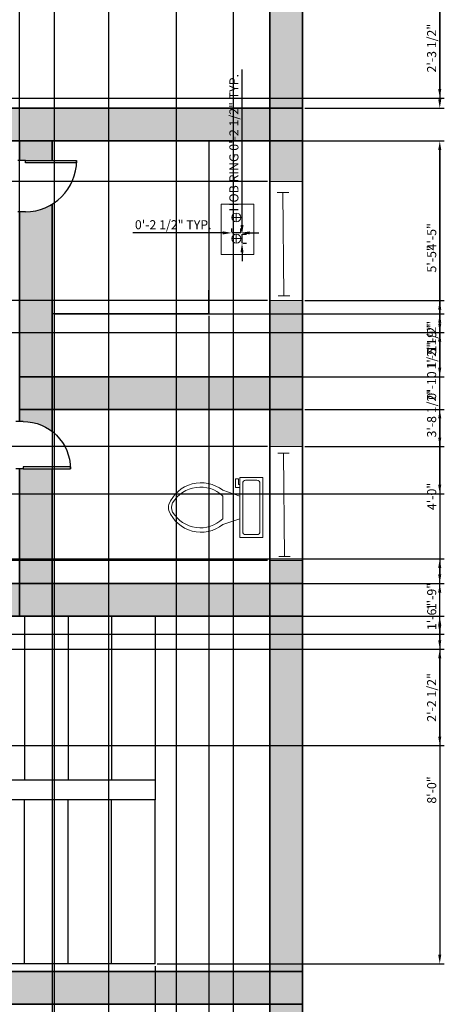
# Model space of a CAD drawing. Units: millimetres. Extents: x 2856 to 3283, y 634 to 1474.
# Tile 7 of 8: x 3165 to 3283, y 1050 to 1321. Entities that reach past the tile are written whole.
import ezdxf

# ---------------------------------------------------------------- set-up
doc = ezdxf.new("R2010")
doc.units = ezdxf.units.MM
for name, color, linetype, lineweight in [('A-ANNO-DIMS', 90, 'Continuous', 18), ('A-EQPM', 140, 'Continuous', 18), ('A-FLOR-CASE', 140, 'Continuous', 25), ('A-FLOR-FIXT', 140, 'Continuous', 18), ('A-WALL-PATT', 2, 'Continuous', 13), ('doors', 10, 'Continuous', 25), ('staircase', 160, 'Continuous', 25), ('walls', 50, 'Continuous', 35), ('windows', 30, 'Continuous', 18)]:
    doc.layers.add(name, color=color, linetype=linetype, lineweight=lineweight)
doc.styles.get("Standard").update_dxf_attribs({"font": 'arial.ttf'})
doc.dimstyles.new('ISO-25', dxfattribs={"dimtxt": 2.5, "dimasz": 2.5, "dimexe": 1.25, "dimexo": 0.625, "dimtad": 1, "dimdec": 0, "dimlunit": 3, "dimtxsty": 'Standard', "dimcen": 2.5, "dimadec": 0, "dimazin": 0, "dimtfac": 1, "dimtdec": 0, "dimtmove": 0, "dimatfit": 3, "dimfxl": 1, "dimarcsym": 0})

# ---------------------------------------------------------------- blocks, each defined once
blk = doc.blocks.new('*U3')
for p, q in [((0, 0), (0, -6)), ((40, 0), (40, -6))]:
    blk.add_line(p, q)
blk.add_lwpolyline([(0, 0), (0, 40), (1.75, 40), (1.75, 0)], close=True)
blk.add_arc((0, 0), 40, 0, 90)
blk = doc.blocks.new('*U6')
for p, q in [((0, 4), (0, 0)), ((36, 4), (36, 0)), ((0, 2), (36, 2))]:
    blk.add_line(p, q)
blk = doc.blocks.new('Toilet - top')
for p, q in [((9.5, -6), (9.5, -2)), ((-10, -8.5), (-8, -8.5)), ((-10, -9.5), (-10, -8.5)), ((-7, -9.5), (-10, -9.5)), ((-8, -8.5), (-8, -8)), ((-7, -8), (-7, -9.5)), ((-4, -8), (-6, -14)), ((4, -8), (6, -14)), ((4, -14), (-4, -14))]:
    blk.add_line(p, q)
blk.add_lwpolyline([(10.5, -8), (10.5, 0), (-10.5, 0), (-10.5, -8)], close=True)
for points in [[(-9.5, -2), (-9.5, -6)], [(8.5, -1), (-8.5, -1)], [(-8.5, -7), (8.5, -7)]]:
    blk.add_lwpolyline(points)
for centre, radius, start, end in [((-8.62, -1.88), 0.884, 81.8699, 188.1301), ((8.62, -1.88), 0.884, 351.8699, 98.1301), ((-8.62, -6.12), 0.884, 171.8699, 278.1301), ((8.62, -6.12), 0.884, 261.8699, 8.1301), ((3.52, -21.58), 12.17, 141.4691, 247.9714), ((4.2, -21.82), 11.33, 136.3677, 238.9468), ((-3.52, -21.58), 12.17, 292.0284, 38.5307), ((-4.2, -21.82), 11.33, 301.053, 43.6321), ((0, -27.88), 4, 245.7318, 294.2682), ((0, -29), 4, 254.8605, 285.1395)]:
    blk.add_arc(centre, radius, start, end)
blk = doc.blocks.new('COOKTOP-BURNER')
for p, q in [((2.45, 1.22), (0, 1.22)), ((1.23, 2.45), (1.23, 0))]:
    blk.add_line(p, q)
blk.add_circle((1.23, 1.22), 1.23)
blk = doc.blocks.new('*D24')
at = {"layer": 'A-ANNO-DIMS', "color": 0, "lineweight": -2, "transparency": 16777216}
for p, q in [((3226.51, 1264.73), (3226.51, 1307.65)), ((3226.51, 1259.78), (3226.51, 1262.23)), ((3226.77, 1262.23), (3227.76, 1262.23)), ((3226.77, 1259.78), (3227.76, 1259.78)), ((3226.51, 1257.28), (3226.51, 1254.78))]:
    blk.add_line(p, q, dxfattribs=at)
at = {"layer": 'A-ANNO-DIMS', "color": 0, "transparency": 16777216}
for points in [[(3226.09, 1264.73), (3226.92, 1264.73), (3226.51, 1262.23)], [(3226.09, 1257.28), (3226.92, 1257.28), (3226.51, 1259.78)]]:
    blk.add_solid(points, dxfattribs=at)
at = {"layer": 'Defpoints', "color": 0, "transparency": 16777216}
for p in [(3226.14, 1262.23), (3226.51, 1262.23), (3226.14, 1259.78)]:
    blk.add_point(p, dxfattribs=at)
at = {"layer": 'A-ANNO-DIMS', "color": 0, "transparency": 16777216, "insert": (3224.59, 1287.44), "char_height": 2.5, "attachment_point": 5, "rotation": 90}
blk.add_mtext('HOB RING 0\'-2 1/2" TYP.', dxfattribs=at)
blk = doc.blocks.new('*D25')
at = {"layer": 'A-ANNO-DIMS', "color": 0, "lineweight": -2, "transparency": 16777216}
for p, q in [((3221.19, 1262.6), (3196.38, 1262.6)), ((3223.69, 1262.86), (3223.69, 1263.85)), ((3226.14, 1262.6), (3223.69, 1262.6)), ((3226.14, 1262.86), (3226.14, 1263.85)), ((3228.64, 1262.6), (3231.14, 1262.6))]:
    blk.add_line(p, q, dxfattribs=at)
at = {"layer": 'A-ANNO-DIMS', "color": 0, "transparency": 16777216}
for points in [[(3221.19, 1263.02), (3221.19, 1262.18), (3223.69, 1262.6)], [(3228.64, 1263.02), (3228.64, 1262.18), (3226.14, 1262.6)]]:
    blk.add_solid(points, dxfattribs=at)
at = {"layer": 'Defpoints', "color": 0, "transparency": 16777216}
for p in [(3223.69, 1262.6), (3223.69, 1262.23), (3226.14, 1262.23)]:
    blk.add_point(p, dxfattribs=at)
at = {"layer": 'A-ANNO-DIMS', "color": 0, "transparency": 16777216, "insert": (3207.53, 1264.52), "char_height": 2.5, "attachment_point": 5}
blk.add_mtext('0\'-2 1/2" TYP.', dxfattribs=at)
blk = doc.blocks.new('*D33')
at = {"layer": 'A-ANNO-DIMS', "color": 0, "lineweight": -2, "transparency": 16777216}
for p, q in [((3073.7, 1014.05), (3073.7, 1470.06)), ((3076.2, 1468.81), (3221.68, 1468.81)), ((3224.18, 1014.05), (3224.18, 1470.06))]:
    blk.add_line(p, q, dxfattribs=at)
at = {"layer": 'A-ANNO-DIMS', "color": 0, "transparency": 16777216}
for points in [[(3076.2, 1469.23), (3076.2, 1468.4), (3073.7, 1468.81)], [(3221.68, 1469.23), (3221.68, 1468.4), (3224.18, 1468.81)]]:
    blk.add_solid(points, dxfattribs=at)
at = {"layer": 'Defpoints', "color": 0, "transparency": 16777216}
for p in [(3224.18, 1468.81), (3073.7, 1013.42), (3224.18, 1013.42)]:
    blk.add_point(p, dxfattribs=at)
at = {"layer": 'A-ANNO-DIMS', "color": 0, "transparency": 16777216, "insert": (3148.94, 1470.73), "char_height": 2.5, "attachment_point": 5}
blk.add_mtext('12\'-6 1/2"', dxfattribs=at)
blk = doc.blocks.new('*D40')
at = {"layer": 'A-ANNO-DIMS', "color": 0, "lineweight": -2, "transparency": 16777216}
for p, q in [((3118.44, 913.07), (3118.44, 1470.06)), ((3120.94, 1468.81), (3172.32, 1468.81)), ((3174.82, 914.65), (3174.82, 1470.06))]:
    blk.add_line(p, q, dxfattribs=at)
at = {"layer": 'A-ANNO-DIMS', "color": 0, "transparency": 16777216}
for points in [[(3120.94, 1469.23), (3120.94, 1468.4), (3118.44, 1468.81)], [(3172.32, 1469.23), (3172.32, 1468.4), (3174.82, 1468.81)]]:
    blk.add_solid(points, dxfattribs=at)
at = {"layer": 'Defpoints', "color": 0, "transparency": 16777216}
for p in [(3174.82, 1468.81), (3118.44, 912.44), (3174.82, 914.03)]:
    blk.add_point(p, dxfattribs=at)
at = {"layer": 'A-ANNO-DIMS', "color": 0, "transparency": 16777216, "insert": (3146.63, 1470.73), "char_height": 2.5, "attachment_point": 5}
blk.add_mtext('4\'-8 1/2"', dxfattribs=at)
blk = doc.blocks.new('*D47')
at = {"layer": 'A-ANNO-DIMS', "color": 0, "lineweight": -2, "transparency": 16777216}
for p, q in [((3243.8, 1430.94), (3282.3, 1430.94)), ((3281.05, 1428.44), (3281.05, 1299.44)), ((3243.8, 1296.94), (3282.3, 1296.94))]:
    blk.add_line(p, q, dxfattribs=at)
at = {"layer": 'A-ANNO-DIMS', "color": 0, "transparency": 16777216}
for points in [[(3280.63, 1428.44), (3281.47, 1428.44), (3281.05, 1430.94)], [(3280.63, 1299.44), (3281.47, 1299.44), (3281.05, 1296.94)]]:
    blk.add_solid(points, dxfattribs=at)
at = {"layer": 'Defpoints', "color": 0, "transparency": 16777216}
for p in [(3243.17, 1430.94), (3243.17, 1296.94), (3281.05, 1296.94)]:
    blk.add_point(p, dxfattribs=at)
at = {"layer": 'A-ANNO-DIMS', "color": 0, "transparency": 16777216, "insert": (3279.17, 1363.94), "char_height": 2.5, "attachment_point": 5, "rotation": 90}
blk.add_mtext('11\'-2"', dxfattribs=at)
blk = doc.blocks.new('*D51')
at = {"layer": 'A-ANNO-DIMS', "color": 0, "lineweight": -2, "transparency": 16777216}
for p, q in [((3165.17, 1223.56), (3165.17, 1470.06)), ((3167.67, 1468.81), (3240.67, 1468.81)), ((3243.17, 1223.56), (3243.17, 1470.06))]:
    blk.add_line(p, q, dxfattribs=at)
at = {"layer": 'A-ANNO-DIMS', "color": 0, "transparency": 16777216}
for points in [[(3167.67, 1469.23), (3167.67, 1468.4), (3165.17, 1468.81)], [(3240.67, 1469.23), (3240.67, 1468.4), (3243.17, 1468.81)]]:
    blk.add_solid(points, dxfattribs=at)
at = {"layer": 'Defpoints', "color": 0, "transparency": 16777216}
for p in [(3243.17, 1468.81), (3165.17, 1222.94), (3243.17, 1222.94)]:
    blk.add_point(p, dxfattribs=at)
at = {"layer": 'A-ANNO-DIMS', "color": 0, "transparency": 16777216, "insert": (3204.17, 1470.71), "char_height": 2.5, "attachment_point": 5}
blk.add_mtext('6\'-6"', dxfattribs=at)
blk = doc.blocks.new('*D52')
at = {"layer": 'A-ANNO-DIMS', "color": 0, "lineweight": -2, "transparency": 16777216}
for p, q in [((3243.8, 1287.94), (3282.3, 1287.94)), ((3281.05, 1285.44), (3281.05, 1225.44)), ((3243.8, 1222.94), (3282.3, 1222.94))]:
    blk.add_line(p, q, dxfattribs=at)
at = {"layer": 'A-ANNO-DIMS', "color": 0, "transparency": 16777216}
for points in [[(3280.63, 1285.44), (3281.47, 1285.44), (3281.05, 1287.94)], [(3280.63, 1225.44), (3281.47, 1225.44), (3281.05, 1222.94)]]:
    blk.add_solid(points, dxfattribs=at)
at = {"layer": 'Defpoints', "color": 0, "transparency": 16777216}
for p in [(3243.17, 1287.94), (3243.17, 1222.94), (3281.05, 1222.94)]:
    blk.add_point(p, dxfattribs=at)
at = {"layer": 'A-ANNO-DIMS', "color": 0, "transparency": 16777216, "insert": (3279.15, 1255.44), "char_height": 2.5, "attachment_point": 5, "rotation": 90}
blk.add_mtext('5\'-5"', dxfattribs=at)
blk = doc.blocks.new('*D53')
at = {"layer": 'A-ANNO-DIMS', "color": 0, "lineweight": -2, "transparency": 16777216}
for p, q in [((3243.8, 1213.94), (3282.3, 1213.94)), ((3281.05, 1211.44), (3281.05, 1168.44)), ((3243.8, 1165.94), (3282.3, 1165.94))]:
    blk.add_line(p, q, dxfattribs=at)
at = {"layer": 'A-ANNO-DIMS', "color": 0, "transparency": 16777216}
for points in [[(3280.63, 1211.44), (3281.47, 1211.44), (3281.05, 1213.94)], [(3280.63, 1168.44), (3281.47, 1168.44), (3281.05, 1165.94)]]:
    blk.add_solid(points, dxfattribs=at)
at = {"layer": 'Defpoints', "color": 0, "transparency": 16777216}
for p in [(3243.17, 1213.94), (3243.17, 1165.94), (3281.05, 1165.94)]:
    blk.add_point(p, dxfattribs=at)
at = {"layer": 'A-ANNO-DIMS', "color": 0, "transparency": 16777216, "insert": (3279.15, 1189.94), "char_height": 2.5, "attachment_point": 5, "rotation": 90}
blk.add_mtext('4\'-0"', dxfattribs=at)
blk = doc.blocks.new('*D54')
at = {"layer": 'A-ANNO-DIMS', "color": 0, "lineweight": -2, "transparency": 16777216}
for p, q in [((3203.14, 1156.94), (3282.3, 1156.94)), ((3281.05, 1154.44), (3281.05, 1063.61)), ((3203.14, 1061.11), (3282.3, 1061.11))]:
    blk.add_line(p, q, dxfattribs=at)
at = {"layer": 'A-ANNO-DIMS', "color": 0, "transparency": 16777216}
for points in [[(3280.63, 1154.44), (3281.47, 1154.44), (3281.05, 1156.94)], [(3280.63, 1063.61), (3281.47, 1063.61), (3281.05, 1061.11)]]:
    blk.add_solid(points, dxfattribs=at)
at = {"layer": 'Defpoints', "color": 0, "transparency": 16777216}
for p in [(3202.52, 1156.94), (3202.52, 1061.11), (3281.05, 1061.11)]:
    blk.add_point(p, dxfattribs=at)
at = {"layer": 'A-ANNO-DIMS', "color": 0, "transparency": 16777216, "insert": (3279.15, 1109.02), "char_height": 2.5, "attachment_point": 5, "rotation": 90}
blk.add_mtext('8\'-0"', dxfattribs=at)
blk = doc.blocks.new('*D55')
at = {"layer": 'A-ANNO-DIMS', "color": 0, "lineweight": -2, "transparency": 16777216}
for p, q in [((3106.52, 1060.48), (3106.52, 634.81)), ((3202.52, 1060.48), (3202.52, 634.81)), ((3109.02, 636.06), (3200.02, 636.06))]:
    blk.add_line(p, q, dxfattribs=at)
at = {"layer": 'A-ANNO-DIMS', "color": 0, "transparency": 16777216}
for points in [[(3109.02, 636.48), (3109.02, 635.65), (3106.52, 636.06)], [(3200.02, 636.48), (3200.02, 635.65), (3202.52, 636.06)]]:
    blk.add_solid(points, dxfattribs=at)
at = {"layer": 'Defpoints', "color": 0, "transparency": 16777216}
for p in [(3106.52, 1061.11), (3202.52, 1061.11), (3202.52, 636.06)]:
    blk.add_point(p, dxfattribs=at)
at = {"layer": 'A-ANNO-DIMS', "color": 0, "transparency": 16777216, "insert": (3154.52, 637.96), "char_height": 2.5, "attachment_point": 5}
blk.add_mtext('8\'-0"', dxfattribs=at)
blk = doc.blocks.new('*D57')
at = {"layer": 'A-ANNO-DIMS', "color": 0, "lineweight": -2, "transparency": 16777216}
for p, q in [((3202.52, 1060.48), (3202.52, 634.81)), ((3243.17, 1058.31), (3243.17, 634.81)), ((3205.02, 636.06), (3240.67, 636.06))]:
    blk.add_line(p, q, dxfattribs=at)
at = {"layer": 'A-ANNO-DIMS', "color": 0, "transparency": 16777216}
for points in [[(3205.02, 636.48), (3205.02, 635.65), (3202.52, 636.06)], [(3240.67, 636.48), (3240.67, 635.65), (3243.17, 636.06)]]:
    blk.add_solid(points, dxfattribs=at)
at = {"layer": 'Defpoints', "color": 0, "transparency": 16777216}
for p in [(3202.52, 1061.11), (3243.17, 1058.94), (3243.17, 636.06)]:
    blk.add_point(p, dxfattribs=at)
at = {"layer": 'A-ANNO-DIMS', "color": 0, "transparency": 16777216, "insert": (3222.85, 637.98), "char_height": 2.5, "attachment_point": 5}
blk.add_mtext('3\'-4 1/2"', dxfattribs=at)
blk = doc.blocks.new('*D65')
at = {"layer": 'A-ANNO-DIMS', "color": 0, "lineweight": -2, "transparency": 16777216}
for p, q in [((3032.03, 1147.82), (3282.3, 1147.82)), ((3281.05, 1123.76), (3281.05, 1145.32)), ((3031.8, 1121.26), (3282.3, 1121.26))]:
    blk.add_line(p, q, dxfattribs=at)
at = {"layer": 'A-ANNO-DIMS', "color": 0, "transparency": 16777216}
for points in [[(3280.63, 1145.32), (3281.47, 1145.32), (3281.05, 1147.82)], [(3280.63, 1123.76), (3281.47, 1123.76), (3281.05, 1121.26)]]:
    blk.add_solid(points, dxfattribs=at)
at = {"layer": 'Defpoints', "color": 0, "transparency": 16777216}
for p in [(3031.41, 1147.82), (3281.05, 1147.82), (3031.17, 1121.26)]:
    blk.add_point(p, dxfattribs=at)
at = {"layer": 'A-ANNO-DIMS', "color": 0, "transparency": 16777216, "insert": (3279.13, 1134.54), "char_height": 2.5, "attachment_point": 5, "rotation": 90}
blk.add_mtext('2\'-2 1/2"', dxfattribs=at)
blk = doc.blocks.new('*D68')
at = {"layer": 'A-ANNO-DIMS', "color": 0, "lineweight": -2, "transparency": 16777216}
for p, q in [((3040.8, 1327.29), (3282.3, 1327.29)), ((3281.05, 1302.28), (3281.05, 1324.79)), ((3040.8, 1299.78), (3282.3, 1299.78))]:
    blk.add_line(p, q, dxfattribs=at)
at = {"layer": 'A-ANNO-DIMS', "color": 0, "transparency": 16777216}
for points in [[(3280.63, 1324.79), (3281.47, 1324.79), (3281.05, 1327.29)], [(3280.63, 1302.28), (3281.47, 1302.28), (3281.05, 1299.78)]]:
    blk.add_solid(points, dxfattribs=at)
at = {"layer": 'Defpoints', "color": 0, "transparency": 16777216}
for p in [(3040.17, 1327.29), (3281.05, 1327.29), (3040.17, 1299.78)]:
    blk.add_point(p, dxfattribs=at)
at = {"layer": 'A-ANNO-DIMS', "color": 0, "transparency": 16777216, "insert": (3279.13, 1313.53), "char_height": 2.5, "attachment_point": 5, "rotation": 90}
blk.add_mtext('2\'-3 1/2"', dxfattribs=at)
blk = doc.blocks.new('*D71')
at = {"layer": 'A-ANNO-DIMS', "color": 0, "lineweight": -2, "transparency": 16777216}
for p, q in [((3150.5, 1421.31), (3150.5, 634.81)), ((3189.65, 1421.31), (3189.65, 634.81)), ((3153, 636.06), (3187.15, 636.06))]:
    blk.add_line(p, q, dxfattribs=at)
at = {"layer": 'A-ANNO-DIMS', "color": 0, "transparency": 16777216}
for points in [[(3153, 636.48), (3153, 635.65), (3150.5, 636.06)], [(3187.15, 636.48), (3187.15, 635.65), (3189.65, 636.06)]]:
    blk.add_solid(points, dxfattribs=at)
at = {"layer": 'Defpoints', "color": 0, "transparency": 16777216}
for p in [(3150.5, 1421.94), (3189.65, 1421.94), (3189.65, 636.06)]:
    blk.add_point(p, dxfattribs=at)
at = {"layer": 'A-ANNO-DIMS', "color": 0, "transparency": 16777216, "insert": (3170.07, 637.97), "char_height": 2.5, "attachment_point": 5}
blk.add_mtext('3\'-3"', dxfattribs=at)
blk = doc.blocks.new('*D73')
at = {"layer": 'A-ANNO-DIMS', "color": 0, "lineweight": -2, "transparency": 16777216}
for p, q in [((2908.8, 1235.12), (3282.3, 1235.12)), ((3281.05, 1193.19), (3281.05, 1232.62)), ((2908.8, 1190.69), (3282.3, 1190.69))]:
    blk.add_line(p, q, dxfattribs=at)
at = {"layer": 'A-ANNO-DIMS', "color": 0, "transparency": 16777216}
for points in [[(3280.63, 1232.62), (3281.47, 1232.62), (3281.05, 1235.12)], [(3280.63, 1193.19), (3281.47, 1193.19), (3281.05, 1190.69)]]:
    blk.add_solid(points, dxfattribs=at)
at = {"layer": 'Defpoints', "color": 0, "transparency": 16777216}
for p in [(2908.17, 1235.12), (3281.05, 1235.12), (2908.17, 1190.69)]:
    blk.add_point(p, dxfattribs=at)
at = {"layer": 'A-ANNO-DIMS', "color": 0, "transparency": 16777216, "insert": (3279.13, 1212.91), "char_height": 2.5, "attachment_point": 5, "rotation": 90}
blk.add_mtext('3\'-8 1/2"', dxfattribs=at)
blk = doc.blocks.new('*D74')
at = {"layer": 'A-ANNO-DIMS', "color": 0, "lineweight": -2, "transparency": 16777216}
for p, q in [((3233.55, 1276.76), (2860.05, 1276.76)), ((2861.3, 1246.44), (2861.3, 1274.26)), ((3233.55, 1243.94), (2860.05, 1243.94))]:
    blk.add_line(p, q, dxfattribs=at)
at = {"layer": 'A-ANNO-DIMS', "color": 0, "transparency": 16777216}
for points in [[(2860.88, 1274.26), (2861.72, 1274.26), (2861.3, 1276.76)], [(2860.88, 1246.44), (2861.72, 1246.44), (2861.3, 1243.94)]]:
    blk.add_solid(points, dxfattribs=at)
at = {"layer": 'Defpoints', "color": 0, "transparency": 16777216}
for p in [(2861.3, 1276.76), (3234.17, 1276.76), (3234.17, 1243.94)]:
    blk.add_point(p, dxfattribs=at)
at = {"layer": 'A-ANNO-DIMS', "color": 0, "transparency": 16777216, "insert": (2859.4, 1260.35), "char_height": 2.5, "attachment_point": 5, "rotation": 90}
blk.add_mtext('2\'-9"', dxfattribs=at)
blk = doc.blocks.new('*D75')
at = {"layer": 'A-ANNO-DIMS', "color": 0, "lineweight": -2, "transparency": 16777216}
for p, q in [((3233.55, 1203.68), (2860.05, 1203.68)), ((2861.3, 1174.81), (2861.3, 1201.18)), ((3233.55, 1172.31), (2860.05, 1172.31))]:
    blk.add_line(p, q, dxfattribs=at)
at = {"layer": 'A-ANNO-DIMS', "color": 0, "transparency": 16777216}
for points in [[(2860.88, 1201.18), (2861.72, 1201.18), (2861.3, 1203.68)], [(2860.88, 1174.81), (2861.72, 1174.81), (2861.3, 1172.31)]]:
    blk.add_solid(points, dxfattribs=at)
at = {"layer": 'Defpoints', "color": 0, "transparency": 16777216}
for p in [(2861.3, 1203.68), (3234.17, 1203.68), (3234.17, 1172.31)]:
    blk.add_point(p, dxfattribs=at)
at = {"layer": 'A-ANNO-DIMS', "color": 0, "transparency": 16777216, "insert": (2859.38, 1188), "char_height": 2.5, "attachment_point": 5, "rotation": 90}
blk.add_mtext('2\'-7 1/2"', dxfattribs=at)
blk = doc.blocks.new('*D79')
at = {"layer": 'A-ANNO-DIMS', "color": 0, "lineweight": -2, "transparency": 16777216}
for p, q in [((2899.8, 1287.94), (3282.3, 1287.94)), ((3281.05, 1237.62), (3281.05, 1285.44)), ((2908.8, 1235.12), (3282.3, 1235.12))]:
    blk.add_line(p, q, dxfattribs=at)
at = {"layer": 'A-ANNO-DIMS', "color": 0, "transparency": 16777216}
for points in [[(3280.63, 1285.44), (3281.47, 1285.44), (3281.05, 1287.94)], [(3280.63, 1237.62), (3281.47, 1237.62), (3281.05, 1235.12)]]:
    blk.add_solid(points, dxfattribs=at)
at = {"layer": 'Defpoints', "color": 0, "transparency": 16777216}
for p in [(2899.17, 1287.94), (3281.05, 1287.94), (2908.17, 1235.12)]:
    blk.add_point(p, dxfattribs=at)
at = {"layer": 'A-ANNO-DIMS', "color": 0, "transparency": 16777216, "insert": (3279.15, 1261.53), "char_height": 2.5, "attachment_point": 5, "rotation": 90}
blk.add_mtext('4\'-5"', dxfattribs=at)
blk = doc.blocks.new('*D80')
at = {"layer": 'A-ANNO-DIMS', "color": 0, "lineweight": -2, "transparency": 16777216}
for p, q in [((3174.17, 1239.69), (3174.17, 634.81)), ((3217.39, 1239.69), (3217.39, 634.81)), ((3176.67, 636.06), (3214.89, 636.06))]:
    blk.add_line(p, q, dxfattribs=at)
at = {"layer": 'A-ANNO-DIMS', "color": 0, "transparency": 16777216}
for points in [[(3176.67, 636.48), (3176.67, 635.65), (3174.17, 636.06)], [(3214.89, 636.48), (3214.89, 635.65), (3217.39, 636.06)]]:
    blk.add_solid(points, dxfattribs=at)
at = {"layer": 'Defpoints', "color": 0, "transparency": 16777216}
for p in [(3174.17, 1240.31), (3217.39, 1240.31), (3217.39, 636.06)]:
    blk.add_point(p, dxfattribs=at)
at = {"layer": 'A-ANNO-DIMS', "color": 0, "transparency": 16777216, "insert": (3195.78, 637.97), "char_height": 2.5, "attachment_point": 5}
blk.add_mtext('3\'-7"', dxfattribs=at)
blk = doc.blocks.new('*D81')
at = {"layer": 'A-ANNO-DIMS', "color": 0, "lineweight": -2, "transparency": 16777216}
for p, q in [((3174.8, 1240.31), (3282.3, 1240.31)), ((3281.05, 1225.44), (3281.05, 1237.81)), ((3165.8, 1222.94), (3282.3, 1222.94))]:
    blk.add_line(p, q, dxfattribs=at)
at = {"layer": 'A-ANNO-DIMS', "color": 0, "transparency": 16777216}
for points in [[(3280.63, 1237.81), (3281.47, 1237.81), (3281.05, 1240.31)], [(3280.63, 1225.44), (3281.47, 1225.44), (3281.05, 1222.94)]]:
    blk.add_solid(points, dxfattribs=at)
at = {"layer": 'Defpoints', "color": 0, "transparency": 16777216}
for p in [(3174.17, 1240.31), (3281.05, 1240.31), (3165.17, 1222.94)]:
    blk.add_point(p, dxfattribs=at)
at = {"layer": 'A-ANNO-DIMS', "color": 0, "transparency": 16777216, "insert": (3279.13, 1231.63), "char_height": 2.5, "attachment_point": 5, "rotation": 90}
blk.add_mtext('1\'-5 1/2"', dxfattribs=at)
blk = doc.blocks.new('*D83')
at = {"layer": 'A-ANNO-DIMS', "color": 0, "lineweight": -2, "transparency": 16777216}
for p, q in [((2951.21, 1172.73), (3282.3, 1172.73)), ((3281.05, 1154.47), (3281.05, 1170.23)), ((2951.21, 1151.97), (3282.3, 1151.97))]:
    blk.add_line(p, q, dxfattribs=at)
at = {"layer": 'A-ANNO-DIMS', "color": 0, "transparency": 16777216}
for points in [[(3280.63, 1170.23), (3281.47, 1170.23), (3281.05, 1172.73)], [(3280.63, 1154.47), (3281.47, 1154.47), (3281.05, 1151.97)]]:
    blk.add_solid(points, dxfattribs=at)
at = {"layer": 'Defpoints', "color": 0, "transparency": 16777216}
for p in [(2950.58, 1172.73), (3281.05, 1172.73), (2950.58, 1151.97)]:
    blk.add_point(p, dxfattribs=at)
at = {"layer": 'A-ANNO-DIMS', "color": 0, "transparency": 16777216, "insert": (3279.15, 1162.35), "char_height": 2.5, "attachment_point": 5, "rotation": 90}
blk.add_mtext('1\'-9"', dxfattribs=at)
blk = doc.blocks.new('*D89')
at = {"layer": 'A-ANNO-DIMS', "color": 0, "lineweight": -2, "transparency": 16777216}
for p, q in [((3031.8, 1165.94), (3282.3, 1165.94)), ((3281.05, 1150.32), (3281.05, 1163.44)), ((3032.03, 1147.82), (3282.3, 1147.82))]:
    blk.add_line(p, q, dxfattribs=at)
at = {"layer": 'A-ANNO-DIMS', "color": 0, "transparency": 16777216}
for points in [[(3280.63, 1163.44), (3281.47, 1163.44), (3281.05, 1165.94)], [(3280.63, 1150.32), (3281.47, 1150.32), (3281.05, 1147.82)]]:
    blk.add_solid(points, dxfattribs=at)
at = {"layer": 'Defpoints', "color": 0, "transparency": 16777216}
for p in [(3031.17, 1165.94), (3281.05, 1165.94), (3031.41, 1147.82)]:
    blk.add_point(p, dxfattribs=at)
at = {"layer": 'A-ANNO-DIMS', "color": 0, "transparency": 16777216, "insert": (3279.15, 1156.88), "char_height": 2.5, "attachment_point": 5, "rotation": 90}
blk.add_mtext('1\'-6"', dxfattribs=at)
blk = doc.blocks.new('*D92')
at = {"layer": 'A-ANNO-DIMS', "color": 0, "lineweight": -2, "transparency": 16777216}
for p, q in [((3208.3, 1343.77), (3208.3, 634.81)), ((3234.17, 1344.54), (3234.17, 634.81)), ((3210.8, 636.06), (3231.67, 636.06))]:
    blk.add_line(p, q, dxfattribs=at)
at = {"layer": 'A-ANNO-DIMS', "color": 0, "transparency": 16777216}
for points in [[(3210.8, 636.48), (3210.8, 635.65), (3208.3, 636.06)], [(3231.67, 636.48), (3231.67, 635.65), (3234.17, 636.06)]]:
    blk.add_solid(points, dxfattribs=at)
at = {"layer": 'Defpoints', "color": 0, "transparency": 16777216}
for p in [(3208.3, 1344.39), (3234.17, 1345.16), (3234.17, 636.06)]:
    blk.add_point(p, dxfattribs=at)
at = {"layer": 'A-ANNO-DIMS', "color": 0, "transparency": 16777216, "insert": (3221.24, 637.94), "char_height": 2.5, "attachment_point": 5}
blk.add_mtext('2\'-2"', dxfattribs=at)
blk = doc.blocks.new('*D96')
at = {"layer": 'A-ANNO-DIMS', "color": 0, "lineweight": -2, "transparency": 16777216}
for p, q in [((3243.8, 1243.94), (3282.3, 1243.94)), ((3281.05, 1225.44), (3281.05, 1241.44)), ((3243.8, 1222.94), (3282.3, 1222.94))]:
    blk.add_line(p, q, dxfattribs=at)
at = {"layer": 'A-ANNO-DIMS', "color": 0, "transparency": 16777216}
for points in [[(3280.63, 1241.44), (3281.47, 1241.44), (3281.05, 1243.94)], [(3280.63, 1225.44), (3281.47, 1225.44), (3281.05, 1222.94)]]:
    blk.add_solid(points, dxfattribs=at)
at = {"layer": 'Defpoints', "color": 0, "transparency": 16777216}
for p in [(3243.17, 1243.94), (3281.05, 1243.94), (3243.17, 1222.94)]:
    blk.add_point(p, dxfattribs=at)
at = {"layer": 'A-ANNO-DIMS', "color": 0, "transparency": 16777216, "insert": (3279.15, 1233.44), "char_height": 2.5, "attachment_point": 5, "rotation": 90}
blk.add_mtext('1\'-9"', dxfattribs=at)
blk = doc.blocks.new('*D97')
at = {"layer": 'A-ANNO-DIMS', "color": 0, "lineweight": -2, "transparency": 16777216}
for p, q in [((3281.05, 1213.94), (3281.05, 1232.1)), ((3243.8, 1213.94), (3282.3, 1213.94)), ((3281.05, 1206.18), (3281.05, 1211.44)), ((3243.8, 1203.68), (3282.3, 1203.68))]:
    blk.add_line(p, q, dxfattribs=at)
at = {"layer": 'A-ANNO-DIMS', "color": 0, "transparency": 16777216}
for points in [[(3280.63, 1211.44), (3281.47, 1211.44), (3281.05, 1213.94)], [(3280.63, 1206.18), (3281.47, 1206.18), (3281.05, 1203.68)]]:
    blk.add_solid(points, dxfattribs=at)
at = {"layer": 'Defpoints', "color": 0, "transparency": 16777216}
for p in [(3243.17, 1213.94), (3281.05, 1213.94), (3243.17, 1203.68)]:
    blk.add_point(p, dxfattribs=at)
at = {"layer": 'A-ANNO-DIMS', "color": 0, "transparency": 16777216, "insert": (3279.13, 1224.27), "char_height": 2.5, "attachment_point": 5, "rotation": 90}
blk.add_mtext('0\'-10 1/2"', dxfattribs=at)

msp = doc.modelspace()

# ---------------------------------------------------------------- hatches: boundary and pattern name
at = {"layer": 'A-WALL-PATT'}
h = msp.add_hatch(color=256, dxfattribs=at)
h.dxf.hatch_style = 1
h.paths.add_polyline_path([(2908.17, 1430.94), (2899.17, 1430.94), (2899.17, 1421.94), (2908.17, 1421.94)])
h.paths.add_polyline_path([(2908.17, 1421.94), (2899.17, 1421.94), (2899.17, 1296.94), (2908.17, 1296.94)])
h.paths.add_polyline_path([(2940.27, 1430.94), (2908.17, 1430.94), (2908.17, 1421.94), (2940.27, 1421.94)])
h.paths.add_polyline_path([(3031.17, 1430.94), (2982.35, 1430.94), (2982.35, 1421.94), (3031.17, 1421.94)])
h.paths.add_polyline_path([(3150.5, 1430.94), (3097.17, 1430.94), (3097.17, 1421.94), (3150.5, 1421.94)])
h.paths.add_polyline_path([(3097.17, 1430.94), (3088.17, 1430.94), (3088.17, 1421.94), (3097.17, 1421.94)])
h.paths.add_polyline_path([(3097.17, 1421.94), (3088.17, 1421.94), (3088.17, 1337.94), (3097.17, 1337.94)])
h.paths.add_polyline_path([(3088.17, 1337.94), (3040.17, 1337.94), (3040.17, 1328.94), (3088.17, 1328.94)])
h.paths.add_polyline_path([(3097.17, 1337.94), (3088.17, 1337.94), (3088.17, 1328.94), (3097.17, 1328.94)])
h.paths.add_polyline_path([(3097.17, 1328.94), (3088.17, 1328.94), (3088.17, 1296.94), (3097.17, 1296.94)])
h.paths.add_polyline_path([(3097.17, 1296.94), (3088.17, 1296.94), (3088.17, 1287.94), (3097.17, 1287.94)])
h.paths.add_polyline_path([(3040.17, 1421.94), (3031.17, 1421.94), (3031.17, 1337.94), (3040.17, 1337.94)])
h.paths.add_polyline_path([(3040.17, 1337.94), (3031.17, 1337.94), (3031.17, 1328.94), (3040.17, 1328.94)])
h.paths.add_polyline_path([(3040.17, 1430.94), (3031.17, 1430.94), (3031.17, 1421.94), (3040.17, 1421.94)])
h.paths.add_polyline_path([(3243.17, 1421.94), (3234.17, 1421.94), (3234.17, 1385.21), (3243.17, 1385.21)])
h.paths.add_polyline_path([(3243.17, 1430.94), (3234.17, 1430.94), (3234.17, 1421.94), (3243.17, 1421.94)])
h.paths.add_polyline_path([(3234.17, 1430.94), (3189.65, 1430.94), (3189.65, 1421.94), (3234.17, 1421.94)])
h.paths.add_polyline_path([(3243.17, 1345.16), (3234.17, 1345.16), (3234.17, 1296.94), (3243.17, 1296.94)])
h.paths.add_polyline_path([(3234.17, 1296.94), (3128.45, 1296.94, -0.06768), (3129.44, 1289.59), (3129.44, 1287.94), (3234.17, 1287.94)])
h.paths.add_polyline_path([(3031.17, 1296.94), (2908.17, 1296.94), (2908.17, 1287.94), (3031.17, 1287.94)])
h.paths.add_polyline_path([(3040.17, 1296.94), (3031.17, 1296.94), (3031.17, 1287.94), (3040.17, 1287.94)])
h.paths.add_polyline_path([(2908.17, 1296.94), (2899.17, 1296.94), (2899.17, 1287.94), (2908.17, 1287.94)])
h.paths.add_polyline_path([(2908.17, 1287.94), (2899.17, 1287.94), (2899.17, 1235.12), (2908.17, 1235.12)])
h.paths.add_polyline_path([(3040.17, 1287.94), (3031.17, 1287.94), (3031.17, 1165.94), (3040.17, 1165.94)])
h.paths.add_polyline_path([(3165.17, 1165.94), (3040.17, 1165.94), (3040.17, 1156.94), (3165.17, 1156.94)])
h.paths.add_polyline_path([(3040.17, 1165.94), (3031.17, 1165.94), (3031.17, 1156.94), (3040.17, 1156.94)])
h.paths.add_polyline_path([(3040.17, 1156.94), (3031.17, 1156.94), (3031.17, 1147.75, -0.068303), (3038.59, 1148.77), (3040.17, 1148.77)])
h.paths.add_polyline_path([(3174.17, 1197.55), (3166.11, 1197.55), (3165.17, 1197.55), (3165.17, 1165.94), (3174.17, 1165.94)])
h.paths.add_polyline_path([(3174.17, 1165.94), (3165.17, 1165.94), (3165.17, 1156.94), (3174.17, 1156.94)])
h.paths.add_polyline_path([(3234.17, 1165.94), (3174.17, 1165.94), (3174.17, 1156.94), (3234.17, 1156.94)])
h.paths.add_polyline_path([(3243.17, 1165.94), (3234.17, 1165.94), (3234.17, 1156.94), (3243.17, 1156.94)])
h.paths.add_polyline_path([(3243.17, 1172.31), (3234.17, 1172.31), (3234.17, 1165.94), (3243.17, 1165.94)])
h.paths.add_polyline_path([(3243.17, 1222.94), (3234.17, 1222.94), (3234.17, 1213.94), (3243.17, 1213.94)])
h.paths.add_polyline_path([(3234.17, 1222.94), (3174.17, 1222.94), (3174.17, 1213.94), (3234.17, 1213.94)])
h.paths.add_polyline_path([(3174.17, 1222.94), (3165.17, 1222.94), (3165.17, 1213.94), (3174.17, 1213.94)])
h.paths.add_polyline_path([(3174.17, 1270.54, -0.139319), (3166.75, 1268.43), (3165.17, 1268.43), (3165.17, 1222.94), (3174.17, 1222.94)])
h.paths.add_polyline_path([(3243.17, 1243.94), (3234.17, 1243.94), (3234.17, 1222.94), (3243.17, 1222.94)])
h.paths.add_polyline_path([(3243.17, 1213.94), (3234.17, 1213.94), (3234.17, 1203.68), (3243.17, 1203.68)])
h.paths.add_polyline_path([(3174.17, 1213.94), (3165.17, 1213.94), (3165.17, 1210.62), (3166.11, 1210.62, -0.16772), (3174.17, 1207.84)])
h.paths.add_polyline_path([(3243.17, 1296.94), (3234.17, 1296.94), (3234.17, 1287.94), (3243.17, 1287.94)])
h.paths.add_polyline_path([(3243.17, 1287.94), (3234.17, 1287.94), (3234.17, 1276.76), (3243.17, 1276.76)])
h.paths.add_polyline_path([(3174.17, 1287.94), (3165.17, 1287.94), (3165.17, 1282.56), (3166.75, 1282.56), (3174.17, 1282.56)])
h.paths.add_polyline_path([(2908.17, 1190.69), (2899.17, 1190.69), (2899.17, 1116.94), (2908.17, 1116.94)])
h.paths.add_polyline_path([(2908.17, 1107.94), (2899.17, 1107.94), (2899.17, 1058.94), (2908.17, 1058.94)])
h.paths.add_polyline_path([(2908.17, 1116.94), (2899.17, 1116.94), (2899.17, 1107.94), (2908.17, 1107.94)])
h.paths.add_polyline_path([(2959.17, 1107.94), (2950.17, 1107.94), (2950.17, 1058.94), (2959.17, 1058.94)])
h.paths.add_polyline_path([(2959.17, 1116.94), (2950.17, 1116.94), (2950.17, 1107.94), (2959.17, 1107.94)])
h.paths.add_polyline_path([(2950.17, 1116.94), (2908.17, 1116.94), (2908.17, 1107.94), (2950.17, 1107.94)])
h.paths.add_polyline_path([(3031.17, 1116.94), (2959.17, 1116.94), (2959.17, 1107.94), (3031.17, 1107.94)])
h.paths.add_polyline_path([(3074.17, 1116.94), (3065.17, 1116.94), (3065.17, 1107.94), (3074.17, 1107.94)])
h.paths.add_polyline_path([(3065.17, 1116.94), (3040.17, 1116.94), (3040.17, 1107.94), (3065.17, 1107.94)])
h.paths.add_polyline_path([(3040.17, 1116.94), (3031.17, 1116.94), (3031.17, 1107.94), (3040.17, 1107.94)])
h.paths.add_polyline_path([(3040.17, 1121.26), (3038.59, 1121.26), (3031.17, 1121.26), (3031.17, 1116.94), (3040.17, 1116.94)])
h.paths.add_polyline_path([(3074.17, 1107.94), (3065.17, 1107.94), (3065.17, 1058.94), (3074.17, 1058.94)])
h.paths.add_polyline_path([(3074.17, 1058.94), (3065.17, 1058.94), (3065.17, 1049.94), (3074.17, 1049.94)])
h.paths.add_polyline_path([(3065.17, 1058.94), (2975.4, 1058.94, -0.174756), (2978.69, 1049.94), (3065.17, 1049.94)])
h.paths.add_polyline_path([(2929.83, 1051.89), (2930.25, 1058.94), (2908.17, 1058.94), (2908.17, 1049.94), (2929.71, 1049.94)])
h.paths.add_polyline_path([(2908.17, 1058.94), (2899.17, 1058.94), (2899.17, 1049.94), (2908.17, 1049.94)])
h.paths.add_polyline_path([(2950.17, 1058.94), (2942.07, 1058.94, -0.146602), (2943.93, 1051.05), (2943.86, 1049.94), (2950.17, 1049.94)])
h.paths.add_polyline_path([(2959.17, 1058.94), (2950.17, 1058.94), (2950.17, 1049.94), (2959.17, 1049.94)])
h.paths.add_polyline_path([(2964.56, 1058.94), (2959.17, 1058.94), (2959.17, 1049.94), (2964.56, 1049.94)])
h.paths.add_polyline_path([(2908.17, 1049.94), (2899.17, 1049.94), (2899.17, 799.94), (2908.17, 799.94)])
h.paths.add_polyline_path([(3234.17, 1058.94), (3074.17, 1058.94), (3074.17, 1049.94), (3234.17, 1049.94)])
h.paths.add_polyline_path([(3243.17, 1156.94), (3234.17, 1156.94), (3234.17, 1058.94), (3243.17, 1058.94)])
h.paths.add_polyline_path([(3243.17, 1058.94), (3234.17, 1058.94), (3234.17, 1049.94), (3243.17, 1049.94)])
h.paths.add_polyline_path([(3243.17, 1049.94), (3234.17, 1049.94), (3234.17, 931.7), (3234.17, 799.94), (3243.17, 799.94), (3243.17, 931.7)])
h.paths.add_polyline_path([(2908.17, 790.94), (2899.17, 790.94), (2899.17, 682.94), (2908.17, 682.94)])
h.paths.add_polyline_path([(2908.17, 799.94), (2899.17, 799.94), (2899.17, 790.94), (2908.17, 790.94)])
h.paths.add_polyline_path([(3234.17, 799.94), (2908.17, 799.94), (2908.17, 790.94), (3234.17, 790.94)])
h.paths.add_polyline_path([(3243.17, 799.94), (3234.17, 799.94), (3234.17, 790.94), (3243.17, 790.94)])
h.paths.add_polyline_path([(3243.17, 790.94), (3234.17, 790.94), (3234.17, 682.94), (3243.17, 682.94)])
h.paths.add_polyline_path([(3234.17, 682.94), (2908.17, 682.94), (2908.17, 673.94), (3234.17, 673.94)])
h.paths.add_polyline_path([(3243.17, 682.94), (3234.17, 682.94), (3234.17, 673.94), (3243.17, 673.94)])
h.paths.add_polyline_path([(2908.17, 682.94), (2899.17, 682.94), (2899.17, 673.94), (2908.17, 673.94)])

# ---------------------------------------------------------------- linework, layer by layer
at = {"layer": 'A-EQPM'}
msp.add_lwpolyline([(3220.73, 1270.53), (3229.76, 1270.53), (3229.76, 1256.61), (3220.73, 1256.61)], close=True, dxfattribs=at)
at = {"layer": 'A-FLOR-CASE'}
for p, q in [((3234.17, 1287.94), (3217.39, 1287.94)), ((3217.39, 1287.94), (3217.39, 1240.31)), ((3217.39, 1240.31), (3217.39, 1246.85)), ((3217.39, 1240.31), (3174.17, 1240.31))]:
    msp.add_line(p, q, dxfattribs=at)
at = {"layer": 'staircase'}
for p, q in [((3166.52, 1156.94), (3166.52, 1111.85)), ((3178.52, 1156.94), (3178.52, 1111.85)), ((3190.52, 1156.94), (3190.52, 1111.85)), ((3202.52, 1156.94), (3202.52, 1106.29)), ((3106.52, 1111.85), (3202.52, 1111.85)), ((3202.52, 1106.29), (3106.06, 1106.29)), ((3166.52, 1061.11), (3166.52, 1106.29)), ((3178.52, 1061.11), (3178.52, 1106.29)), ((3190.52, 1061.11), (3190.52, 1106.29)), ((3202.52, 1061.11), (3202.52, 1106.29)), ((3202.52, 1061.11), (3106.06, 1061.11))]:
    msp.add_line(p, q, dxfattribs=at)
at = {"layer": 'walls'}
for p, q in [((3234.17, 1430.94), (3234.17, 1287.94)), ((3243.17, 1430.94), (3243.17, 1287.94)), ((3128.45, 1296.94), (3243.17, 1296.94)), ((3129.44, 1287.94), (3243.17, 1287.94)), ((3165.17, 1287.94), (3165.17, 1282.56)), ((3174.17, 1287.94), (3174.17, 1282.56)), ((3234.17, 1287.94), (3234.17, 931.7)), ((3243.17, 1287.94), (3243.17, 931.7)), ((3174.17, 1270.54), (3174.17, 1207.84)), ((3165.17, 1268.43), (3165.17, 1210.62)), ((3165.17, 1222.94), (3243.17, 1222.94)), ((3165.17, 1213.94), (3243.17, 1213.94)), ((3165.17, 1197.55), (3165.17, 1156.94)), ((3174.17, 1197.55), (3174.17, 1156.94)), ((3031.17, 1165.94), (3243.17, 1165.94)), ((3031.17, 1156.94), (3243.17, 1156.94)), ((2975.4, 1058.94), (3243.17, 1058.94)), ((2978.69, 1049.94), (3243.17, 1049.94))]:
    msp.add_line(p, q, dxfattribs=at)
at = {"layer": 'windows'}
for p, q in [((3234.17, 1276.76), (3243.17, 1276.76)), ((3243.17, 1243.94), (3234.17, 1243.94)), ((3243.17, 1203.68), (3234.17, 1203.68)), ((3243.17, 1172.31), (3234.17, 1172.31))]:
    msp.add_line(p, q, dxfattribs=at)

# ---------------------------------------------------------------- block references
at = {"layer": 'A-EQPM'}
msp.add_blockref('COOKTOP-BURNER', (3223.69, 1265.63), dxfattribs=at)
at = {"layer": 'A-EQPM', "rotation": 90.00000000003192}
msp.add_blockref('COOKTOP-BURNER', (3226.14, 1259.78), dxfattribs=at)
at = {"layer": 'A-FLOR-FIXT', "xscale": 0.7880357630815594, "yscale": 0.7880357630815594, "zscale": 0.7880357630815594, "rotation": 270}
msp.add_blockref('Toilet - top', (3232.21, 1186.91), dxfattribs=at)
at = {"layer": 'doors', "rotation": 270}
for p, xscale, yscale, zscale in [((3166.75, 1282.56), 0.3532068763098237, 0.3532068763098237, 0.3532068763098237), ((3166.11, 1197.55), -0.3267993458683955, 0.3267993458683955, 0.3267993458683955)]:
    msp.add_blockref('*U3', p, dxfattribs=dict(at, xscale=xscale, yscale=yscale, zscale=zscale))
at = {"layer": 'windows', "xscale": 0.7908534711778109, "yscale": 0.7908534711778109, "zscale": 0.7908534711778109, "rotation": 90.56209262617526}
for p in [(3239.66, 1245.29), (3239.78, 1173.41)]:
    msp.add_blockref('*U6', p, dxfattribs=at)

# ---------------------------------------------------------------- dimensions: what is measured, and where the dimension line sits
at = {"layer": 'A-ANNO-DIMS'}
for base, p1, p2, picture, middle in [((3224.18, 1468.81), (3073.7, 1013.42), (3224.18, 1013.42), '*D33', (3148.94, 1470.73)), ((3174.82, 1468.81), (3118.44, 912.44), (3174.82, 914.03), '*D40', (3146.63, 1470.73)), ((3243.17, 1468.81), (3165.17, 1222.94), (3243.17, 1222.94), '*D51', (3204.17, 1470.71)), ((3189.6495, 636.0634), (3150.4985, 1421.9396), (3189.6495, 1421.9396), '*D71', (3170.074, 637.9657)), ((3234.17, 636.06), (3208.3, 1344.39), (3234.17, 1345.16), '*D92', (3221.24, 637.94)), ((3217.39, 636.06), (3174.17, 1240.31), (3217.39, 1240.31), '*D80', (3195.78, 637.97)), ((3202.52, 636.06), (3106.52, 1061.11), (3202.52, 1061.11), '*D55', (3154.52, 637.96)), ((3243.1743, 636.0634), (3202.518, 1061.1095), (3243.1743, 1058.9396), '*D57', (3222.8462, 637.9819))]:
    dim = msp.add_linear_dim(base=base, p1=p1, p2=p2, dimstyle='ISO-25', override={"dimdec": 1, "dimlfac": 1, "dimrnd": 0, "dimzin": 1, "dimdsep": 46, "dimlunit": 4, "dimfrac": 2}, dxfattribs=at)
    dim.commit()
    dim.dimension.update_dxf_attribs({"geometry": picture, "text_midpoint": middle})
for base, p1, p2, picture, middle in [((3281.05, 1296.94), (3243.17, 1430.94), (3243.17, 1296.94), '*D47', (3279.17, 1363.94)), ((3281.05, 1327.29), (3040.17, 1299.78), (3040.17, 1327.29), '*D68', (3279.13, 1313.53)), ((3281.05, 1287.94), (2908.17, 1235.12), (2899.17, 1287.94), '*D79', (3279.15, 1261.53)), ((3281.05, 1222.94), (3243.17, 1287.94), (3243.17, 1222.94), '*D52', (3279.15, 1255.44)), ((2861.3, 1276.76), (3234.17, 1243.94), (3234.17, 1276.76), '*D74', (2859.4, 1260.35)), ((3281.05, 1243.94), (3243.17, 1222.94), (3243.17, 1243.94), '*D96', (3279.15, 1233.44)), ((3281.05, 1240.31), (3165.17, 1222.94), (3174.17, 1240.31), '*D81', (3279.13, 1231.63)), ((3281.05, 1235.12), (2908.17, 1190.69), (2908.17, 1235.12), '*D73', (3279.13, 1212.91)), ((3281.05, 1213.94), (3243.17, 1203.68), (3243.17, 1213.94), '*D97', (3279.13, 1224.27)), ((3281.05, 1165.94), (3243.17, 1213.94), (3243.17, 1165.94), '*D53', (3279.15, 1189.94)), ((2861.3, 1203.68), (3234.17, 1172.31), (3234.17, 1203.68), '*D75', (2859.38, 1188)), ((3281.05, 1172.73), (2950.58, 1151.97), (2950.58, 1172.73), '*D83', (3279.15, 1162.35)), ((3281.05, 1165.94), (3031.41, 1147.82), (3031.17, 1165.94), '*D89', (3279.15, 1156.88)), ((3281.05, 1061.11), (3202.52, 1156.94), (3202.52, 1061.11), '*D54', (3279.15, 1109.02)), ((3281.05, 1147.82), (3031.17, 1121.26), (3031.41, 1147.82), '*D65', (3279.13, 1134.54))]:
    dim = msp.add_linear_dim(base=base, p1=p1, p2=p2, angle=90, dimstyle='ISO-25', override={"dimdec": 1, "dimlfac": 1, "dimrnd": 0, "dimzin": 1, "dimdsep": 46, "dimlunit": 4, "dimfrac": 2}, dxfattribs=at)
    dim.commit()
    dim.dimension.update_dxf_attribs({"geometry": picture, "text_midpoint": middle})
for base, p1, p2, angle, text, picture, middle in [((3226.5076, 1262.2329), (3226.1401, 1259.7823), (3226.1401, 1262.2329), 90, 'HOB RING <> TYP.', '*D24', (3224.5892, 1287.4426)), ((3223.6895, 1262.6005), (3226.1401, 1262.2329), (3223.6895, 1262.2329), 180, '<> TYP.', '*D25', (3207.5324, 1264.5181))]:
    dim = msp.add_linear_dim(base=base, p1=p1, p2=p2, angle=angle, text=text, dimstyle='ISO-25', override={"dimdec": 1, "dimlfac": 1, "dimrnd": 0, "dimzin": 1, "dimdsep": 46, "dimlunit": 4, "dimfrac": 2}, dxfattribs=at)
    dim.commit()
    dim.dimension.update_dxf_attribs({"geometry": picture, "text_midpoint": middle})

doc.saveas('drawing.dxf')
